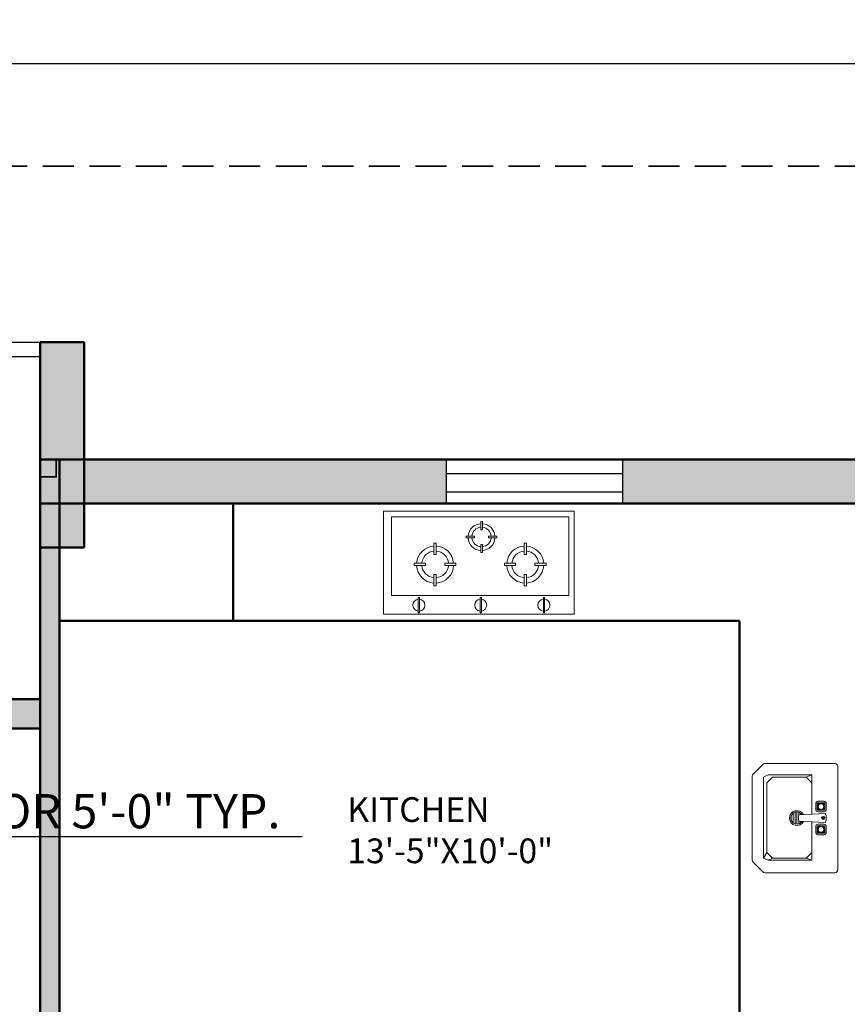
# Model space of a CAD drawing. Units: inches. Extents: x -7 to 1228, y -146 to 1091.
# Tile 76 of 88: x 376 to 545, y 890 to 1091. Entities that reach past the tile are written whole.
import ezdxf

# ---------------------------------------------------------------- set-up
doc = ezdxf.new("R2010")
doc.units = ezdxf.units.IN
doc.linetypes.add('DASHED2', pattern=[9.525, 6.35, -3.175])
for name, color, linetype, lineweight in [('A-ANNO-DIMS', 2, 'Continuous', 18), ('A-AREA-IDEN', 7, 'Continuous', 18), ('A-COLS', 6, 'Continuous', 35), ('A-FURN', 8, 'Continuous', 18), ('A-GLAZ', 175, 'Continuous', 25), ('A-WALL', 7, 'Continuous', 50), ('A-WALL-PATT', 251, 'Continuous', 13), ('C-PROP', 1, 'DASHED2', 35)]:
    doc.layers.add(name, color=color, linetype=linetype, lineweight=lineweight)
doc.styles.get("Standard").update_dxf_attribs({"font": 'arial.ttf'})
doc.dimstyles.new('ISO-25', dxfattribs={"dimtxt": 7, "dimasz": 4, "dimexe": 1.25, "dimexo": 0.625, "dimtad": 1, "dimdec": 1, "dimlunit": 3, "dimtxsty": 'Standard', "dimcen": 2.5, "dimadec": 0, "dimazin": 0, "dimtfac": 1, "dimtdec": 1, "dimtmove": 1, "dimatfit": 3, "dimfxl": 1, "dimarcsym": 0})

# ---------------------------------------------------------------- blocks, each defined once
blk = doc.blocks.new('A$C72243D80')
at = {"ltscale": 1000}
for p, q in [((0, 0), (0, 384.2)), ((0, 384.2), (712, 384.2)), ((712, 384.2), (712, 0)), ((29.5, 68.9), (29.5, 363.2)), ((29.5, 363.2), (692.7, 363.2)), ((363.5, 314.5), (363.5, 345.1)), ((363.5, 345.1), (369.5, 345.1)), ((369.5, 345.1), (369.5, 314.5)), ((692.7, 363.2), (692.7, 68.9)), ((369.5, 314.5), (363.5, 314.5)), ((188.1, 264.2), (188.1, 222.1)), ((196.4, 264.2), (188.1, 264.2)), ((196.4, 222.1), (196.4, 264.2)), ((309.4, 291), (340, 291)), ((309.4, 285), (309.4, 291)), ((340, 285), (309.4, 285)), ((340, 291), (340, 285)), ((363.5, 260), (363.5, 229.4)), ((369.5, 260), (363.5, 260)), ((369.5, 229.4), (369.5, 260)), ((392.3, 291), (392.3, 285)), ((422.9, 291), (392.3, 291)), ((392.3, 285), (422.9, 285)), ((422.9, 285), (422.9, 291)), ((525.9, 222.1), (525.9, 264.2)), ((525.9, 264.2), (534.1, 264.2)), ((534.1, 264.2), (534.1, 222.1)), ((188.1, 222.1), (196.4, 222.1)), ((363.5, 229.4), (369.5, 229.4)), ((534.1, 222.1), (525.9, 222.1)), ((114.7, 189.8), (156.8, 189.8)), ((114.7, 181.6), (114.7, 189.8)), ((156.8, 189.8), (156.8, 181.6)), ((228.6, 189.8), (228.6, 181.6)), ((270.7, 189.8), (228.6, 189.8)), ((270.7, 181.6), (270.7, 189.8)), ((451.5, 189.8), (493.6, 189.8)), ((451.5, 181.6), (451.5, 189.8)), ((493.6, 189.8), (493.6, 181.6)), ((565.5, 189.8), (565.5, 181.6)), ((607.6, 189.8), (565.5, 189.8)), ((607.6, 181.6), (607.6, 189.8)), ((156.8, 181.6), (114.7, 181.6)), ((188.1, 147.2), (196.4, 147.2)), ((188.1, 105.1), (188.1, 147.2)), ((196.4, 147.2), (196.4, 105.1)), ((228.6, 181.6), (270.7, 181.6)), ((493.6, 181.6), (451.5, 181.6)), ((525.9, 147.2), (525.9, 105.1)), ((534.1, 147.2), (525.9, 147.2)), ((534.1, 105.1), (534.1, 147.2)), ((565.5, 181.6), (607.6, 181.6)), ((196.4, 105.1), (188.1, 105.1)), ((525.9, 105.1), (534.1, 105.1)), ((692.7, 68.9), (29.5, 68.9)), ((129.6, 61.1), (129.6, 5)), ((134.4, 61.1), (129.6, 61.1)), ((134.4, 5), (134.4, 61.1)), ((360.9, 5), (360.9, 61.1)), ((360.9, 61.1), (365.7, 61.1)), ((365.7, 61.1), (365.7, 5)), ((597, 5), (597, 61.1)), ((597, 61.1), (601.8, 61.1)), ((601.8, 61.1), (601.8, 5)), ((712, 0), (0, 0)), ((129.6, 5), (134.4, 5)), ((365.7, 5), (360.9, 5)), ((601.8, 5), (597, 5))]:
    blk.add_line(p, q, dxfattribs=at)
for centre, radius, start, end in [((366.2, 287.2), 50.3, 93.0344, 175.7271), ((366.2, 287.2), 50.3, 4.2729, 86.1838), ((366.1, 287.8), 36.3, 94.0374, 175.0142), ((366.1, 287.8), 36.3, 4.9858, 84.5356), ((366.2, 287.2), 50.3, 182.5783, 266.9656), ((366.1, 287.8), 36.3, 184.5153, 265.9626), ((366.1, 287.8), 36.3, 275.4644, 355.4847), ((366.2, 287.2), 50.3, 273.8162, 357.4217), ((192.7, 184.7), 69.2, 93.8162, 175.7271), ((192.9, 185.5), 49.9, 95.4644, 175.0142), ((192.7, 184.7), 69.2, 4.2729, 86.9656), ((192.9, 185.5), 49.9, 4.9858, 85.9626), ((529.5, 184.7), 69.2, 93.0344, 175.7271), ((529.4, 185.5), 49.9, 94.0374, 175.0142), ((529.5, 184.7), 69.2, 4.2729, 86.1838), ((529.4, 185.5), 49.9, 4.9858, 84.5356), ((192.7, 184.7), 69.2, 182.5783, 266.1838), ((192.9, 185.5), 49.9, 184.5153, 264.5356), ((192.9, 185.5), 49.9, 274.0374, 355.4847), ((192.7, 184.7), 69.2, 273.0344, 357.4217), ((529.5, 184.7), 69.2, 182.5783, 266.9656), ((529.4, 185.5), 49.9, 184.5153, 265.9626), ((529.5, 184.7), 69.2, 273.8162, 357.4217), ((529.4, 185.5), 49.9, 275.4644, 355.4847), ((132.3, 33.2), 22.5, 96.7453, 263.2547), ((132.3, 33.2), 22.5, 275.4789, 84.5211), ((363.1, 33.2), 22.5, 95.4789, 264.5211), ((363.1, 33.2), 22.5, 276.7453, 83.2547), ((599.2, 33.2), 22.5, 95.4789, 264.5211), ((599.2, 33.2), 22.5, 276.7453, 83.2547)]:
    blk.add_arc(centre, radius, start, end, dxfattribs=at)
blk = doc.blocks.new('A$C4CB854FF')
for p, q in [((0, 0.3675), (0, 0.0552)), ((0.4725, 0.38), (0.0125, 0.38)), ((0.485, 0.0552), (0.485, 0.3675)), ((0.1677, 0.2932), (0.1677, 0.318)), ((0.1745, 0.2919), (0.1745, 0.3194)), ((0.1773, 0.3221), (0.2048, 0.3221)), ((0.1787, 0.329), (0.2034, 0.329)), ((0.2075, 0.3194), (0.2075, 0.2919)), ((0.2144, 0.318), (0.2144, 0.2932)), ((0.2279, 0.2104), (0.2213, 0.3235)), ((0.2337, 0.329), (0.2502, 0.329)), ((0.2625, 0.3235), (0.256, 0.2104)), ((0.2694, 0.318), (0.2694, 0.2932)), ((0.2763, 0.3194), (0.2763, 0.2919)), ((0.3065, 0.3221), (0.279, 0.3221)), ((0.3052, 0.329), (0.2804, 0.329)), ((0.3093, 0.2919), (0.3093, 0.3194)), ((0.3162, 0.2932), (0.3162, 0.318)), ((0.05, 0.265), (0.2247, 0.265)), ((0.06, 0.24), (0.05, 0.265)), ((0.05, 0.07), (0.05, 0.265)), ((0.085, 0.265), (0.06, 0.24)), ((0.2048, 0.2891), (0.1773, 0.2891)), ((0.2034, 0.2822), (0.1787, 0.2822)), ((0.2591, 0.265), (0.43, 0.265)), ((0.279, 0.2891), (0.3065, 0.2891)), ((0.2804, 0.2822), (0.3052, 0.2822)), ((0.395, 0.265), (0.42, 0.24)), ((0.42, 0.24), (0.43, 0.265)), ((0.43, 0.07), (0.43, 0.265)), ((0.06, 0.24), (0.06, 0.09)), ((0.42, 0.24), (0.42, 0.09)), ((0.2152, 0.1984), (0.2694, 0.1984)), ((0.2297, 0.2066), (0.2165, 0.2066)), ((0.2681, 0.1901), (0.2165, 0.1901)), ((0.2272, 0.2149), (0.2208, 0.2149)), ((0.2638, 0.1819), (0.2208, 0.1819)), ((0.2505, 0.2052), (0.2334, 0.2052)), ((0.2681, 0.2066), (0.2541, 0.2066)), ((0.2638, 0.2149), (0.2566, 0.2149)), ((0.2533, 0.1736), (0.2313, 0.1736)), ((0.06, 0.09), (0.085, 0.065)), ((0.42, 0.09), (0.395, 0.065)), ((0.42, 0.09), (0.43, 0.07)), ((0.0037, 0.0463), (0.0463, 0.0037)), ((0.05, 0.07), (0.06, 0.05)), ((0.42, 0.05), (0.06, 0.05)), ((0.085, 0.065), (0.395, 0.065)), ((0.395, 0.065), (0.42, 0.05)), ((0.43, 0.07), (0.42, 0.05)), ((0.4387, 0.0037), (0.4813, 0.0463)), ((0.0552, 0), (0.4298, 0))]:
    blk.add_line(p, q)
for centre, radius in [((0.191, 0.3056), 0.0165), ((0.191, 0.3056), 0.0127), ((0.2419, 0.3152), 0.00688), ((0.2419, 0.3152), 0.00344), ((0.2928, 0.3056), 0.0165), ((0.2928, 0.3056), 0.0127)]:
    blk.add_circle(centre, radius)
for centre, radius, start, end in [((0.0125, 0.3675), 0.0125, 90, 180), ((0.4725, 0.3675), 0.0125, 0, 90), ((0.1787, 0.318), 0.011, 90, 180), ((0.1773, 0.3194), 0.00275, 90, 180), ((0.2034, 0.318), 0.011, 0, 90), ((0.2048, 0.3194), 0.00275, 360, 90), ((0.2329, 0.314), 0.015, 87.1975, 140.7274), ((0.2509, 0.314), 0.015, 39.2726, 92.8025), ((0.2804, 0.318), 0.011, 90, 180), ((0.279, 0.3194), 0.00275, 90, 180), ((0.3052, 0.318), 0.011, 0, 90), ((0.3065, 0.3194), 0.00275, 360, 90), ((0.1787, 0.2932), 0.011, 180, 270), ((0.1773, 0.2919), 0.00275, 180, 270), ((0.2034, 0.2932), 0.011, 270, 0), ((0.2048, 0.2919), 0.00275, 270, 0), ((0.2804, 0.2932), 0.011, 180, 270), ((0.279, 0.2919), 0.00275, 180, 270), ((0.3052, 0.2932), 0.011, 270, 360), ((0.3065, 0.2919), 0.00275, 270, 0), ((0.2423, 0.1984), 0.033, 118.6883, 62.8686), ((0.2423, 0.1984), 0.0271, 124.7758, 57.2247), ((0.2334, 0.2107), 0.0055, 183.3274, 270), ((0.2505, 0.2107), 0.0055, 270, 356.6726), ((0.0125, 0.0552), 0.0125, 180, 225), ((0.4725, 0.0552), 0.0125, 315, 0), ((0.0552, 0.0125), 0.0125, 225, 270), ((0.4298, 0.0125), 0.0125, 270, 315)]:
    blk.add_arc(centre, radius, start, end)
blk = doc.blocks.new('*D11')
at = {"layer": 'A-ANNO-DIMS', "color": 0, "lineweight": -2, "transparency": 16777216}
for p, q in [((0, 1061.62), (0, 1083.25)), ((4, 1082), (1183, 1082)), ((1187, 1061.62), (1187, 1083.25))]:
    blk.add_line(p, q, dxfattribs=at)
at = {"layer": 'A-ANNO-DIMS', "color": 0, "transparency": 16777216}
for points in [[(4, 1082.67), (4, 1081.33), (0, 1082)], [(1183, 1082.67), (1183, 1081.33), (1187, 1082)]]:
    blk.add_solid(points, dxfattribs=at)
at = {"layer": 'Defpoints', "color": 0, "transparency": 16777216}
for p in [(1187, 1082), (0, 1061), (1187, 1061)]:
    blk.add_point(p, dxfattribs=at)
at = {"layer": 'A-ANNO-DIMS', "color": 0, "transparency": 16777216, "insert": (593.5, 1086.2), "char_height": 7, "attachment_point": 5}
blk.add_mtext('98\'-11"', dxfattribs=at)
blk = doc.blocks.new('WIN-36')
for p, q in [((0, 36), (0, 0)), ((9, 36), (0, 36)), ((2.34, 36), (2.34, 0)), ((6.14, 0), (6.14, 36)), ((9, 0), (9, 36)), ((0, 0), (9, 0)), ((2.34, 0), (6.14, 0))]:
    blk.add_line(p, q)
blk = doc.blocks.new('*D52')
at = {"layer": 'A-ANNO-DIMS', "color": 0, "lineweight": -2, "transparency": 16777216}
for p, q in [((274.55, 945.37), (274.55, 935.75)), ((334.55, 945.37), (334.55, 935.75)), ((278.55, 937), (330.55, 937)), ((304.55, 937), (308.46, 923.95)), ((308.46, 923.95), (433.58, 923.95))]:
    blk.add_line(p, q, dxfattribs=at)
at = {"layer": 'A-ANNO-DIMS', "color": 0, "transparency": 16777216}
for points in [[(278.55, 937.67), (278.55, 936.33), (274.55, 937)], [(330.55, 937.67), (330.55, 936.33), (334.55, 937)]]:
    blk.add_solid(points, dxfattribs=at)
at = {"layer": 'Defpoints', "color": 0, "transparency": 16777216}
for p in [(274.55, 946), (334.55, 946), (334.55, 937)]:
    blk.add_point(p, dxfattribs=at)
at = {"layer": 'A-ANNO-DIMS', "color": 0, "transparency": 16777216, "insert": (371.02, 928.19), "char_height": 7, "attachment_point": 5}
blk.add_mtext('BALCONY DOOR 5\'-0" TYP.', dxfattribs=at)

msp = doc.modelspace()

# ---------------------------------------------------------------- hatches: boundary and pattern name
at = {"layer": 'A-COLS'}
h = msp.add_hatch(color=256, dxfattribs=at)
h.dxf.hatch_style = 1
h.paths.add_polyline_path([(380, 983), (389, 983), (389, 1001), (383.29, 1001), (383.29, 997.45), (380, 997.45)])
h = msp.add_hatch(color=256, dxfattribs=at)
h.dxf.hatch_style = 1
h.paths.add_polyline_path([(383.29, 997.45), (383.29, 1001), (380, 1001), (380, 997.45)])
at = {"layer": 'A-WALL-PATT'}
h = msp.add_hatch(color=256, dxfattribs=at)
h.dxf.hatch_style = 1
h.paths.add_polyline_path([(69, 568), (60, 568), (60, 493), (63.29, 493), (69, 493)])
h.paths.add_polyline_path([(69, 662.41), (60, 662.41), (60, 586), (69, 586)], flags=17)
h.paths.add_polyline_path([(69, 723), (184, 723), (184, 734), (179, 734), (179, 728), (69, 728), (69, 741.62), (60, 741.62), (60, 698.41), (69, 698.41)], flags=17)
h.paths.add_polyline_path([(69, 782), (231, 782), (231, 728), (231, 723), (231, 586), (236, 586), (236, 787), (69, 787), (69, 800.13), (60, 800.13), (60, 765.62), (69, 765.62)])
h.paths.add_polyline_path([(184, 842), (189, 842), (189, 848), (173, 848), (173, 842), (179, 842), (179, 787), (184, 787)])
h.paths.add_polyline_path([(118.22, 69), (69, 69), (69, 60), (118.22, 60)])
h.paths.add_polyline_path([(227, 69), (154.22, 69), (154.22, 60), (227, 60)])
h.paths.add_polyline_path([(236, 60), (232.71, 60), (227, 60), (227, 36), (236, 36)])
h.paths.add_polyline_path([(389, 60), (380, 60), (380, 36), (389, 36)])
h.paths.add_polyline_path([(384, 181), (380, 181), (380, 115), (380, 78), (384, 78)])
h.paths.add_polyline_path([(380, 115), (334.55, 115), (334.55, 109), (380, 109)])
h.paths.add_polyline_path([(274.55, 115), (236, 115), (236, 201), (232.71, 201), (231, 201), (231, 78), (236, 78), (236, 109), (274.55, 109)])
h.paths.add_polyline_path([(69, 123), (60, 123), (60, 78), (69, 78)])
h.paths.add_polyline_path([(69, 201), (60, 201), (60, 159), (69, 159)])
h.paths.add_polyline_path([(143, 219), (69, 219), (69, 213), (143, 213)], flags=17)
h.paths.add_polyline_path([(189, 219), (184, 219), (184, 274), (231, 274), (231, 219), (236, 219), (236, 279), (184, 279), (184, 297), (179, 297), (179, 279), (69, 279), (69, 290.91), (60, 290.91), (60, 262.18), (69, 262.18), (69, 274), (179, 274), (179, 219), (173, 219), (173, 213), (189, 213)])
h.paths.add_polyline_path([(69, 238.18), (60, 238.18), (60, 219), (69, 219)], flags=17)
h.paths.add_polyline_path([(69, 333), (60, 333), (60, 314.91), (69, 314.91), (69, 316.96)])
h.paths.add_polyline_path([(190, 338), (184, 338), (69, 338), (69, 333), (179, 333), (179, 327), (184, 327), (184, 333.02), (190, 333.05)])
h.paths.add_polyline_path([(69, 386.81), (60, 386.81), (60, 351), (69, 351)])
h.paths.add_polyline_path([(69, 475), (60, 475), (60, 422.81), (69, 422.81)])
h.paths.add_polyline_path([(236, 475), (231, 475), (231, 351.24), (236, 351.24)])
h.paths.add_polyline_path([(384, 475), (380, 475), (380, 362), (384, 362)])
h.paths.add_polyline_path([(547, 307), (439, 307), (439, 356), (445, 356), (445, 362), (433, 362), (433, 307), (380, 307), (380, 244), (380, 241), (384, 241), (384, 301), (433, 301), (433, 277), (439, 277), (439, 301), (547, 301)])
h.paths.add_polyline_path([(547, 241), (439, 241), (439, 247), (433, 247), (433, 235), (547, 235)])
h.paths.add_polyline_path([(450, 69), (440.29, 69), (424.89, 69), (389, 69), (389, 60), (450, 60)])
h.paths.add_polyline_path([(547, 69), (486, 69), (486, 60), (547, 60)])
h.paths.add_polyline_path([(556, 148.27), (547, 148.27), (547, 78), (556, 78)])
h.paths.add_polyline_path([(556, 223), (547, 223), (547, 195), (547, 184.27), (556, 184.27)])
h.paths.add_polyline_path([(556, 311.19), (547, 311.19), (547, 273.08), (556, 273.08)])
h.paths.add_polyline_path([(556, 344), (552.71, 344), (547, 344), (547, 335.19), (556, 335.19)])
h.paths.add_polyline_path([(556, 249.08), (547, 249.08), (547, 241), (556, 241)])
h.paths.add_polyline_path([(547, 362), (475, 362), (475, 356), (547, 356)], flags=0)
h.paths.add_polyline_path([(556, 399.62), (547, 399.62), (547, 362), (556, 362)])
h.paths.add_polyline_path([(556, 475), (547, 475), (547, 435.62), (556, 435.62)])
h.paths.add_polyline_path([(547, 493), (389, 493), (389, 487), (547, 487)])
h.paths.add_polyline_path([(380, 493), (278, 493), (278, 487), (380, 487)])
h.paths.add_polyline_path([(227, 493), (69, 493), (69, 487), (227, 487)])
h.paths.add_polyline_path([(643, 122.44), (634, 122.44), (634, 78), (643, 78)])
h.paths.add_polyline_path([(702.5, 69), (692.79, 69), (677.39, 69), (643, 69), (643, 60), (702.5, 60)])
h.paths.add_polyline_path([(798, 69), (738.5, 69), (738.5, 60), (798, 60)])
h.paths.add_polyline_path([(807, 60), (803.71, 60), (798, 60), (798, 36), (807, 36)])
h.paths.add_polyline_path([(807, 109), (846.75, 109), (846.75, 115), (807, 115), (807, 159), (802, 159), (802, 78), (807, 78)])
h.paths.add_polyline_path([(807, 201), (802, 201), (802, 195), (807, 195)])
h.paths.add_polyline_path([(643, 201), (634, 201), (634, 158.44), (643, 158.44)])
h.paths.add_polyline_path([(756, 225), (751, 225), (751, 219), (643, 219), (643, 213), (756, 213)])
h.paths.add_polyline_path([(643, 240.85), (634, 240.85), (634, 219), (643, 219)])
h.paths.add_polyline_path([(643, 274), (643, 288.63), (634, 288.63), (634, 264.85), (643, 264.85)])
h.paths.add_polyline_path([(802, 279), (756, 279), (756, 297), (751, 297), (751, 279), (643, 279), (643, 274), (751, 274), (751, 255), (756, 255), (756, 274), (802, 274)])
h.paths.add_polyline_path([(807, 333), (803.71, 333), (802, 333), (802, 279), (802, 274), (802, 219), (807, 219)])
h.paths.add_polyline_path([(956, 182), (951, 182), (951, 115), (906.75, 115), (906.75, 109), (951, 109), (951, 78), (956, 78)])
h.paths.add_polyline_path([(960, 60), (951, 60), (951, 36), (960, 36)])
h.paths.add_polyline_path([(1021, 69), (1005.78, 69), (960, 69), (960, 60), (1021, 60)])
h.paths.add_polyline_path([(956, 224), (951, 224), (951, 218), (956, 218)])
h.paths.add_polyline_path([(956, 302), (1004, 302), (1004, 278), (1010, 278), (1010, 302), (1118, 302), (1118, 290.81), (1127, 290.81), (1127, 326.97), (1118, 326.97), (1118, 320.97), (1118, 307), (1010, 307), (1010, 356), (1016, 356), (1016, 362), (1004, 362), (1004, 307), (951, 307), (951, 244), (951, 242), (954.29, 242), (956, 242)])
h.paths.add_polyline_path([(643, 333), (634, 333), (634, 312.63), (643, 312.63), (643, 316.96)])
h.paths.add_polyline_path([(756, 338), (643, 338), (643, 333), (751, 333), (751, 327), (756, 327)])
h.paths.add_polyline_path([(643, 388), (634, 388), (634, 351), (643, 351)])
h.paths.add_polyline_path([(807, 357), (802, 357), (802, 351), (807, 351)])
h.paths.add_polyline_path([(807, 475), (802, 475), (802, 393), (807, 393)])
h.paths.add_polyline_path([(643, 475), (634, 475), (634, 424), (643, 424)])
h.paths.add_polyline_path([(798, 493), (643, 493), (643, 487), (798, 487)])
h.paths.add_polyline_path([(634, 493), (556, 493), (556, 487), (634, 487)])
h.paths.add_polyline_path([(813, 493), (807, 493), (807, 487), (813, 487)])
h.paths.add_polyline_path([(951, 493), (849, 493), (849, 487), (951, 487)])
h.paths.add_polyline_path([(956, 484), (951, 484), (951, 374), (956, 374)])
h.paths.add_polyline_path([(1109, 493), (969, 493), (969, 487), (1109, 487)])
h.paths.add_polyline_path([(1127, 484), (1118, 484), (1118, 450.64), (1127, 450.64)])
h.paths.add_polyline_path([(1127, 414.64), (1118, 414.64), (1118, 365), (1127, 365)])
h.paths.add_polyline_path([(1109, 362), (1046, 362), (1046, 356), (1109, 356)], flags=17)
h.paths.add_polyline_path([(1127, 356), (1123.45, 356), (1118, 356), (1118, 350.97), (1127, 350.97)], flags=0)
h.paths.add_polyline_path([(1127, 266.81), (1118, 266.81), (1118, 262.36), (1118, 242), (1127, 242)], flags=17)
h.paths.add_polyline_path([(1118, 242), (1010, 242), (1010, 248), (1004, 248), (1004, 237), (1118, 237)])
h.paths.add_polyline_path([(1127, 224), (1118, 224), (1118, 170), (1127, 170)])
h.paths.add_polyline_path([(1127, 134), (1118, 134), (1118, 78), (1127, 78)])
h.paths.add_polyline_path([(1118, 69), (1057, 69), (1057, 60), (1118, 60)])
h.paths.add_polyline_path([(227, 571.55), (227, 574), (69, 574), (69, 568), (227, 568)])
h.paths.add_polyline_path([(380, 571.55), (380, 574), (278, 574), (278, 568), (380, 568)])
h.paths.add_polyline_path([(242, 574), (236, 574), (236, 568), (242, 568)])
h.paths.add_polyline_path([(547, 571.55), (547, 574), (389, 574), (389, 568), (547, 568)])
h.paths.add_polyline_path([(384, 733), (380, 733), (380, 586), (384, 586)])
h.paths.add_polyline_path([(556, 646), (634, 646), (634, 655), (547, 655), (547, 586), (556, 586)])
h.paths.add_polyline_path([(634, 574), (556, 574), (556, 568), (634, 568)])
h.paths.add_polyline_path([(643, 655), (634, 655), (634, 586), (643, 586)])
h.paths.add_polyline_path([(798, 574), (643, 574), (643, 568), (798, 568)])
h.paths.add_polyline_path([(643, 663.85), (634, 663.85), (634, 655), (643, 655)])
h.paths.add_polyline_path([(556, 676.97), (547, 676.97), (547, 655), (556, 655)])
h.paths.add_polyline_path([(556, 733), (547, 733), (547, 712.97), (556, 712.97)])
h.paths.add_polyline_path([(643, 710), (634, 710), (634, 699.85), (643, 699.85)])
h.paths.add_polyline_path([(807, 668), (802, 668), (802, 586), (807, 586)])
h.paths.add_polyline_path([(951, 574), (849, 574), (849, 568), (951, 568)])
h.paths.add_polyline_path([(956, 691), (951, 691), (951, 577), (956, 577)])
h.paths.add_polyline_path([(1109, 574), (969, 574), (969, 568), (1109, 568)])
h.paths.add_polyline_path([(1127, 643.4), (1118, 643.4), (1118, 577), (1127, 577)])
h.paths.add_polyline_path([(1127, 568), (1123.45, 568), (1118, 568), (1118, 493), (1127, 493)])
h.paths.add_polyline_path([(1127, 733), (1118, 733), (1118, 679.4), (1127, 679.4)])
h.paths.add_polyline_path([(1127, 777.35), (1118, 777.35), (1118, 770.04), (1118, 751), (1127, 751)], flags=17)
h.paths.add_polyline_path([(1118, 751), (1010, 751), (1010, 757), (1004, 757), (1004, 745), (1118, 745)])
h.paths.add_polyline_path([(956, 811), (1004, 811), (1004, 787), (1010, 787), (1010, 811), (1017.87, 811), (1017.87, 811.63, -0.414214), (1018.25, 812), (1031.98, 812, -0.414214), (1032.35, 811.63), (1032.35, 811), (1118, 811), (1118, 801.35), (1127, 801.35), (1127, 834.69), (1118, 834.69), (1118, 830.24), (1118, 817), (1010, 817), (1010, 866), (1016, 866), (1016, 872), (1004, 872), (1004, 817), (956, 817), (956, 866), (951, 866), (951, 751), (954.29, 751), (956, 751)])
h.paths.add_polyline_path([(1118, 872), (1046, 872), (1046, 866), (1118, 866)], flags=17)
h.paths.add_polyline_path([(1127, 924.71), (1118, 924.71), (1118, 884), (1127, 884)])
h.paths.add_polyline_path([(1127, 866), (1123.71, 866), (1118, 866), (1118, 858.69), (1127, 858.69)], flags=17)
h.paths.add_polyline_path([(956, 983), (951, 983), (951, 952), (807, 952), (807, 983), (802, 983), (802, 902), (807, 902), (807, 946), (951, 946), (951, 884), (956, 884)])
h.paths.add_polyline_path([(807, 842), (802, 842), (802, 787), (756, 787), (756, 806), (751, 806), (751, 787), (643, 787), (643, 782), (751, 782), (751, 764), (756, 764), (756, 782), (802, 782), (802, 728), (807, 728)])
h.paths.add_polyline_path([(756, 848), (643, 848), (643, 842), (751, 842), (751, 836), (756, 836)])
h.paths.add_polyline_path([(756, 734), (751, 734), (751, 728), (643, 728), (643, 723), (756, 723)])
h.paths.add_polyline_path([(643, 749.79), (634, 749.79), (634, 728), (637.29, 728), (643, 728)])
h.paths.add_polyline_path([(643, 805.41), (634, 805.41), (634, 773.79), (643, 773.79)])
h.paths.add_polyline_path([(643, 896.66), (634, 896.66), (634, 860), (637.29, 860), (643, 860)])
h.paths.add_polyline_path([(643, 842), (634, 842), (634, 829.41), (643, 829.41)])
h.paths.add_polyline_path([(643, 983), (634, 983), (634, 932.66), (643, 932.66)])
h.paths.add_polyline_path([(1127, 983), (1118, 983), (1118, 960.71), (1127, 960.71)])
h.paths.add_polyline_path([(1118, 1001), (1077.53, 1001), (1077.53, 992), (1118, 992)])
h.paths.add_polyline_path([(1041.53, 1001), (960, 1001), (960, 992), (1041.53, 992)])
h.paths.add_polyline_path([(960, 1025), (951, 1025), (951, 1001), (954.29, 1001), (960, 1001)])
h.paths.add_polyline_path([(807, 1025), (798, 1025), (798, 1001), (807, 1001)])
h.paths.add_polyline_path([(798, 1001), (738.5, 1001), (738.5, 992), (798, 992)])
h.paths.add_polyline_path([(702.5, 1001), (643, 1001), (643, 992), (702.5, 992)])
h.paths.add_polyline_path([(547, 1001), (499.11, 1001), (499.11, 992), (547, 992)])
h.paths.add_polyline_path([(463.11, 1001), (389, 1001), (389, 992), (463.11, 992)])
h.paths.add_polyline_path([(389, 1025), (380, 1025), (380, 1022), (380, 1001), (383.29, 1001), (389, 1001)])
h.paths.add_polyline_path([(236, 1025), (227, 1025), (227, 1001), (236, 1001)])
h.paths.add_polyline_path([(236, 983), (231, 983), (231, 860), (236, 860)])
h.paths.add_polyline_path([(274.55, 952), (236, 952), (236, 946), (274.55, 946)])
h.paths.add_polyline_path([(380, 952), (334.55, 952), (334.55, 946), (380, 946)])
h.paths.add_polyline_path([(384, 983), (380, 983), (380, 884), (383.29, 884), (384, 884)])
h.paths.add_polyline_path([(227, 1001), (155.01, 1001), (155.01, 992), (162.87, 992), (227, 992)])
h.paths.add_polyline_path([(119.01, 1001), (69, 1001), (69, 992), (119.01, 992)])
h.paths.add_polyline_path([(69, 983), (60, 983), (60, 922.99), (69, 922.99)])
h.paths.add_polyline_path([(69, 886.99), (60, 886.99), (60, 860), (63.29, 860), (69, 860)])
h.paths.add_polyline_path([(143, 848), (69, 848), (69, 842), (143, 842)])

# ---------------------------------------------------------------- linework, layer by layer
at = {"layer": 'A-COLS'}
msp.add_lwpolyline([(380, 1001), (383.29, 1001), (383.29, 997.45), (380, 997.45)], close=True, dxfattribs=at)
at = {"layer": 'A-GLAZ'}
for p, q in [((236, 1025), (380, 1025)), ((380, 1022), (236, 1022))]:
    msp.add_line(p, q, dxfattribs=at)
at = {"layer": 'A-WALL'}
for p, q in [((380, 1001), (380, 1025)), ((380, 1025), (389, 1025)), ((380, 1025), (380, 1022)), ((389, 1025), (389, 1001)), ((380, 1001), (380, 866)), ((380, 1001), (389, 1001)), ((380, 983), (380, 1001)), ((556, 1001), (380, 1001)), ((384, 1001), (384, 866)), ((389, 1001), (389, 983)), ((556, 992), (380, 992)), ((419.46, 968), (419.46, 992)), ((389, 983), (380, 983)), ((523, 968), (384, 968)), ((523, 968), (523, 872)), ((380, 952), (236, 952)), ((380, 946), (236, 946))]:
    msp.add_line(p, q, dxfattribs=at)
at = {"layer": 'C-PROP'}
msp.add_line((1187, 1061), (0, 1061), dxfattribs=at)

# ---------------------------------------------------------------- block references
at = {"layer": 'A-FURN', "xscale": 0.0547573419986423, "yscale": 0.0547573419986423, "zscale": 0.0547573419986423}
msp.add_blockref('A$C72243D80', (450.21, 969.42), dxfattribs=at)
at = {"layer": 'A-FURN', "xscale": 45.99182974636398, "yscale": 45.99182974636398, "zscale": 45.99182974636398, "rotation": 270}
msp.add_blockref('A$C4CB854FF', (525.62, 938.83), dxfattribs=at)
at = {"layer": 'A-GLAZ', "extrusion": (0, 0, -1), "zscale": -1, "rotation": 90.00000000000003}
msp.add_blockref('WIN-36', (-463.11, 992), dxfattribs=at)

# ---------------------------------------------------------------- texts
at = {"layer": 'A-AREA-IDEN', "insert": (441.27, 931.95), "char_height": 5.0568, "attachment_point": 1}
msp.add_mtext_dynamic_manual_height_columns(' KITCHEN\\P 13\'-5"X10\'-0"', width=137.2821, gutter_width=25.28, heights=[0], dxfattribs=at)

# ---------------------------------------------------------------- dimensions: what is measured, and where the dimension line sits
at = {"layer": 'A-ANNO-DIMS'}
dim = msp.add_linear_dim(base=(1187, 1082), p1=(0, 1061), p2=(1187, 1061), dimstyle='ISO-25', override={"dimclrd": 0, "dimclre": 0, "dimclrt": 0}, dxfattribs=at)
dim.commit()
dim.dimension.update_dxf_attribs({"geometry": '*D11', "text_midpoint": (593.5, 1086.2)})
dim = msp.add_linear_dim(base=(334.55, 937), p1=(274.55, 946), p2=(334.55, 946), text='BALCONY DOOR <> TYP.', dimstyle='ISO-25', override={"dimdec": 1, "dimlfac": 1, "dimrnd": 0, "dimzin": 1, "dimdsep": 46, "dimlunit": 4, "dimfrac": 2}, dxfattribs=at)
dim.commit()
dim.dimension.update_dxf_attribs({"geometry": '*D52', "text_midpoint": (309.09, 928.19)})

doc.saveas('drawing.dxf')
